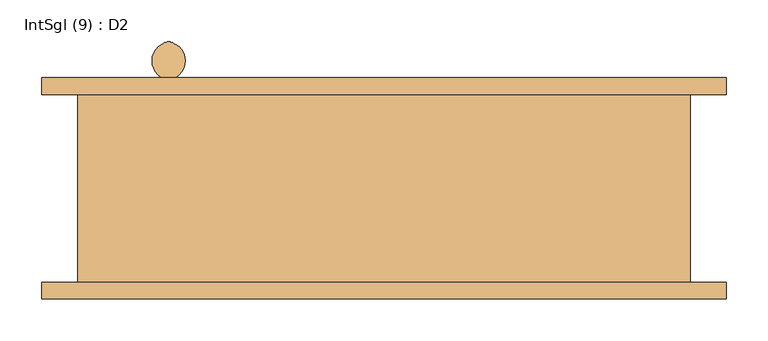
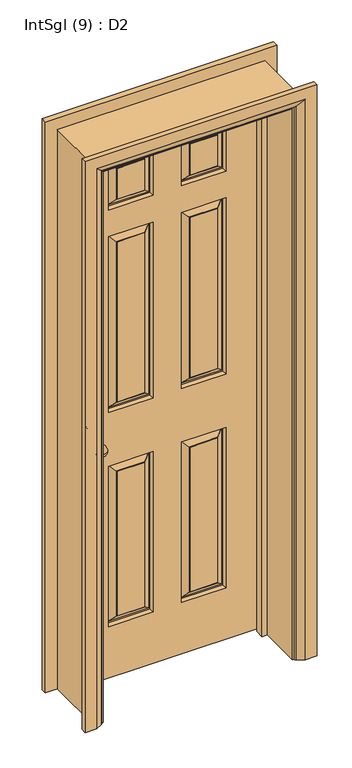
"""IFC4 building model written with IfcOpenShell, lengths in millimetres: door geometry, IntSgl (9) : D2."""

from ifc_helpers import new_model, si_unit, point, frame, origin, place, context, project, spatial, polyline, circle_curve, ellipse_curve, trimmed, outline, extrude, faceted_brep, source, transform, mapped, element, save
from ifc_brep_helpers import plane_surface, cylinder_surface, revolved_surface, advanced_brep


def intsgl_9_d2_5357b631(model_context):
    return source(origin(), model_context, "Body", "SolidModel", [
        advanced_brep(
        [(-253.0, 55.5, 900.0), (-258.0, 11.062589, 900.0), (-263.0, 55.5, 900.0), (-263.0, 70.5, 900.0), (-253.0, 70.5, 900.0), (-278.0, 74.5, 900.0), (-238.0, 74.5, 900.0), (-278.0, 70.5, 900.0), (-238.0, 70.5, 900.0)],
        [
            (0, 1, circle_curve(frame((-261.1884862, 33.9213505, 900.0), z_axis=(0.0, 0.0, -1.0), x_axis=(0.0, 1.0, 0.0)), 23.0800654)),
            (1, 2, circle_curve(frame((-254.8115138, 33.9213505, 900.0), z_axis=(0.0, 0.0, -1.0), x_axis=(0.0, 1.0, 0.0)), 23.0800654)),
            (2, 0, circle_curve(frame((-258.0, 55.5, 900.0), z_axis=(0.0, -1.0, 0.0), x_axis=(-1.0, 0.0, 0.0)), 5.0)),
            (0, 2, circle_curve(frame((-258.0, 55.5, 900.0), z_axis=(0.0, -1.0, 0.0), x_axis=(-1.0, 0.0, 0.0)), 5.0)),
            (2, 3),
            (3, 4, circle_curve(frame((-258.0, 70.5, 900.0), z_axis=(0.0, -1.0, 0.0), x_axis=(-1.0, 0.0, 0.0)), 5.0)),
            (4, 0),
            (4, 3, circle_curve(frame((-258.0, 70.5, 900.0), z_axis=(0.0, -1.0, 0.0), x_axis=(-1.0, 0.0, 0.0)), 5.0)),
            (5, 6, circle_curve(frame((-258.0, 74.5, 900.0), z_axis=(0.0, 1.0, 0.0), x_axis=(1.0, 0.0, 0.0)), 20.0)),
            (6, 5, circle_curve(frame((-258.0, 74.5, 900.0), z_axis=(0.0, 1.0, 0.0), x_axis=(1.0, 0.0, 0.0)), 20.0)),
            (7, 8, circle_curve(frame((-258.0, 70.5, 900.0), z_axis=(0.0, -1.0, 0.0), x_axis=(1.0, 0.0, 0.0)), 20.0)),
            (8, 7, circle_curve(frame((-258.0, 70.5, 900.0), z_axis=(0.0, -1.0, 0.0), x_axis=(1.0, 0.0, 0.0)), 20.0)),
            (6, 8),
            (7, 5),
        ],
        [
            revolved_surface(trimmed(ellipse_curve(frame((-254.8115138, 33.9213505, 900.0), z_axis=(0.0, 0.0, -1.0), x_axis=(0.0, 1.0, 0.0)), 23.0800654, 23.0800654), [point((-258.0, 11.062589, 900.0))], [point((-263.0, 55.5, 900.0))], True, "CARTESIAN"), (-258.0, 70.5, 900.0), (0.0, 1.0, 0.0)),
            cylinder_surface(frame((-258.0, 70.5, 900.0), z_axis=(0.0, 1.0, 0.0), x_axis=(-1.0, 0.0, 0.0)), 5.0),
            plane_surface(frame((-238.0, 74.5, 900.0), z_axis=(0.0, 1.0, 0.0), x_axis=(0.0, 0.0, 1.0))),
            plane_surface(frame((-238.0, 70.5, 900.0), z_axis=(0.0, -1.0, 0.0), x_axis=(0.0, 0.0, -1.0))),
            cylinder_surface(frame((-258.0, 70.5, 900.0), z_axis=(0.0, 1.0, 0.0), x_axis=(1.0, 0.0, 0.0)), 20.0),
        ],
        [
            (0, [[1, 2, 3]]),
            (0, [[-1, 4, -2]]),
            (1, [[5, 6, 7, -3]]),
            (1, [[-7, 8, -5, -4]]),
            (2, [[9, 10]]),
            (3, [[11, 12], [-8, -6]]),
            (4, [[13, -11, 14, -10]]),
            (4, [[-14, -12, -13, -9]]),
        ],
    ),
        advanced_brep(
        [(-253.0, 131.5, 900.0), (-263.0, 131.5, 900.0), (-258.0, 175.937411, 900.0), (-253.0, 116.5, 900.0), (-263.0, 116.5, 900.0), (-278.0, 112.5, 900.0), (-238.0, 112.5, 900.0), (-278.0, 116.5, 900.0), (-238.0, 116.5, 900.0)],
        [
            (0, 1, circle_curve(frame((-258.0, 131.5, 900.0), z_axis=(0.0, 1.0, 0.0), x_axis=(-1.0, 0.0, 0.0)), 5.0)),
            (1, 2, circle_curve(frame((-254.8115138, 153.0786495, 900.0), z_axis=(0.0, 0.0, -1.0), x_axis=(0.0, -1.0, 0.0)), 23.0800654)),
            (2, 0, circle_curve(frame((-261.1884862, 153.0786495, 900.0), z_axis=(0.0, 0.0, -1.0), x_axis=(0.0, -1.0, 0.0)), 23.0800654)),
            (1, 0, circle_curve(frame((-258.0, 131.5, 900.0), z_axis=(0.0, 1.0, 0.0), x_axis=(-1.0, 0.0, 0.0)), 5.0)),
            (0, 3),
            (3, 4, circle_curve(frame((-258.0, 116.5, 900.0), z_axis=(0.0, 1.0, 0.0), x_axis=(-1.0, 0.0, 0.0)), 5.0)),
            (4, 1),
            (4, 3, circle_curve(frame((-258.0, 116.5, 900.0), z_axis=(0.0, 1.0, 0.0), x_axis=(-1.0, 0.0, 0.0)), 5.0)),
            (5, 6, circle_curve(frame((-258.0, 112.5, 900.0), z_axis=(0.0, -1.0, 0.0), x_axis=(1.0, 0.0, 0.0)), 20.0)),
            (6, 5, circle_curve(frame((-258.0, 112.5, 900.0), z_axis=(0.0, -1.0, 0.0), x_axis=(1.0, 0.0, 0.0)), 20.0)),
            (7, 8, circle_curve(frame((-258.0, 116.5, 900.0), z_axis=(0.0, 1.0, 0.0), x_axis=(1.0, 0.0, 0.0)), 20.0)),
            (8, 7, circle_curve(frame((-258.0, 116.5, 900.0), z_axis=(0.0, 1.0, 0.0), x_axis=(1.0, 0.0, 0.0)), 20.0)),
            (5, 7),
            (8, 6),
        ],
        [
            revolved_surface(trimmed(ellipse_curve(frame((-254.8115138, 153.0786495, 900.0), z_axis=(0.0, 0.0, 1.0), x_axis=(0.0, -1.0, 0.0)), 23.0800654, 23.0800654), [point((-258.0, 175.937411, 900.0))], [point((-263.0, 131.5, 900.0))], True, "CARTESIAN"), (-258.0, 116.5, 900.0), (0.0, -1.0, 0.0)),
            cylinder_surface(frame((-258.0, 116.5, 900.0), z_axis=(0.0, -1.0, 0.0), x_axis=(-1.0, 0.0, 0.0)), 5.0),
            plane_surface(frame((-238.0, 112.5, 900.0), z_axis=(0.0, -1.0, 0.0), x_axis=(0.0, 0.0, 1.0))),
            plane_surface(frame((-238.0, 116.5, 900.0), z_axis=(0.0, 1.0, 0.0), x_axis=(0.0, 0.0, -1.0))),
            cylinder_surface(frame((-258.0, 116.5, 900.0), z_axis=(0.0, -1.0, 0.0), x_axis=(1.0, 0.0, 0.0)), 20.0),
        ],
        [
            (0, [[1, 2, 3]]),
            (0, [[-2, 4, -3]]),
            (1, [[-1, 5, 6, 7]]),
            (1, [[-4, -7, 8, -5]]),
            (2, [[9, 10]]),
            (3, [[11, 12], [-6, -8]]),
            (4, [[-9, 13, -12, 14]]),
            (4, [[-10, -14, -11, -13]]),
        ],
    ),
        faceted_brep([(-333.0, 74.5, 2058.0), (-333.0, 74.5, 8.0), (333.0, 74.5, 8.0), (333.0, 74.5, 2058.0), (-50.0, 74.5, 800.0), (-50.0, 74.5, 200.0), (-208.0, 74.5, 200.0), (-208.0, 74.5, 800.0), (208.0, 74.5, 800.0), (208.0, 74.5, 200.0), (50.0, 74.5, 200.0), (50.0, 74.5, 800.0), (-50.0, 74.5, 1658.0), (-50.0, 74.5, 1000.0), (-208.0, 74.5, 1000.0), (-208.0, 74.5, 1658.0), (208.0, 74.5, 1658.0), (208.0, 74.5, 1000.0), (50.0, 74.5, 1000.0), (50.0, 74.5, 1658.0), (-50.0, 74.5, 1933.0), (-50.0, 74.5, 1758.0), (-208.0, 74.5, 1758.0), (-208.0, 74.5, 1933.0), (208.0, 74.5, 1933.0), (208.0, 74.5, 1758.0), (50.0, 74.5, 1758.0), (50.0, 74.5, 1933.0), (-80.0, 74.5, 230.0), (-80.0, 74.5, 770.0), (-178.0, 74.5, 770.0), (-178.0, 74.5, 230.0), (178.0, 74.5, 230.0), (178.0, 74.5, 770.0), (80.0, 74.5, 770.0), (80.0, 74.5, 230.0), (-80.0, 74.5, 1030.0), (-80.0, 74.5, 1628.0), (-178.0, 74.5, 1628.0), (-178.0, 74.5, 1030.0), (178.0, 74.5, 1030.0), (178.0, 74.5, 1628.0), (80.0, 74.5, 1628.0), (80.0, 74.5, 1030.0), (-80.0, 74.5, 1788.0), (-80.0, 74.5, 1903.0), (-178.0, 74.5, 1903.0), (-178.0, 74.5, 1788.0), (178.0, 74.5, 1788.0), (178.0, 74.5, 1903.0), (80.0, 74.5, 1903.0), (80.0, 74.5, 1788.0), (-333.0, 112.5, 2058.0), (333.0, 112.5, 2058.0), (333.0, 112.5, 8.0), (-333.0, 112.5, 8.0), (50.0, 112.5, 800.0), (50.0, 112.5, 200.0), (208.0, 112.5, 200.0), (208.0, 112.5, 800.0), (-208.0, 112.5, 800.0), (-208.0, 112.5, 200.0), (-50.0, 112.5, 200.0), (-50.0, 112.5, 800.0), (50.0, 112.5, 1658.0), (50.0, 112.5, 1000.0), (208.0, 112.5, 1000.0), (208.0, 112.5, 1658.0), (-208.0, 112.5, 1658.0), (-208.0, 112.5, 1000.0), (-50.0, 112.5, 1000.0), (-50.0, 112.5, 1658.0), (50.0, 112.5, 1933.0), (50.0, 112.5, 1758.0), (208.0, 112.5, 1758.0), (208.0, 112.5, 1933.0), (-208.0, 112.5, 1933.0), (-208.0, 112.5, 1758.0), (-50.0, 112.5, 1758.0), (-50.0, 112.5, 1933.0), (80.0, 112.5, 230.0), (80.0, 112.5, 770.0), (178.0, 112.5, 770.0), (178.0, 112.5, 230.0), (-178.0, 112.5, 230.0), (-178.0, 112.5, 770.0), (-80.0, 112.5, 770.0), (-80.0, 112.5, 230.0), (80.0, 112.5, 1030.0), (80.0, 112.5, 1628.0), (178.0, 112.5, 1628.0), (178.0, 112.5, 1030.0), (-178.0, 112.5, 1030.0), (-178.0, 112.5, 1628.0), (-80.0, 112.5, 1628.0), (-80.0, 112.5, 1030.0), (80.0, 112.5, 1788.0), (80.0, 112.5, 1903.0), (178.0, 112.5, 1903.0), (178.0, 112.5, 1788.0), (-178.0, 112.5, 1788.0), (-178.0, 112.5, 1903.0), (-80.0, 112.5, 1903.0), (-80.0, 112.5, 1788.0), (80.0, 111.5, 230.0), (80.0, 111.5, 770.0), (58.0, 97.5, 208.0), (58.0, 97.5, 792.0), (78.0, 111.5, 772.0), (78.0, 111.5, 228.0), (53.0, 97.5, 797.0), (53.0, 97.5, 203.0), (178.0, 111.5, 770.0), (200.0, 97.5, 792.0), (180.0, 111.5, 772.0), (205.0, 97.5, 797.0), (178.0, 111.5, 230.0), (200.0, 97.5, 208.0), (180.0, 111.5, 228.0), (205.0, 97.5, 203.0), (-178.0, 111.5, 230.0), (-178.0, 111.5, 770.0), (-200.0, 97.5, 208.0), (-200.0, 97.5, 792.0), (-180.0, 111.5, 772.0), (-180.0, 111.5, 228.0), (-205.0, 97.5, 797.0), (-205.0, 97.5, 203.0), (-80.0, 111.5, 770.0), (-58.0, 97.5, 792.0), (-78.0, 111.5, 772.0), (-53.0, 97.5, 797.0), (-80.0, 111.5, 230.0), (-58.0, 97.5, 208.0), (-78.0, 111.5, 228.0), (-53.0, 97.5, 203.0), (80.0, 111.5, 1030.0), (80.0, 111.5, 1628.0), (58.0, 97.5, 1008.0), (58.0, 97.5, 1650.0), (78.0, 111.5, 1630.0), (78.0, 111.5, 1028.0), (53.0, 97.5, 1655.0), (53.0, 97.5, 1003.0), (178.0, 111.5, 1628.0), (200.0, 97.5, 1650.0), (180.0, 111.5, 1630.0), (205.0, 97.5, 1655.0), (178.0, 111.5, 1030.0), (200.0, 97.5, 1008.0), (180.0, 111.5, 1028.0), (205.0, 97.5, 1003.0), (-178.0, 111.5, 1030.0), (-178.0, 111.5, 1628.0), (-200.0, 97.5, 1008.0), (-200.0, 97.5, 1650.0), (-180.0, 111.5, 1630.0), (-180.0, 111.5, 1028.0), (-205.0, 97.5, 1655.0), (-205.0, 97.5, 1003.0), (-80.0, 111.5, 1628.0), (-58.0, 97.5, 1650.0), (-78.0, 111.5, 1630.0), (-53.0, 97.5, 1655.0), (-80.0, 111.5, 1030.0), (-58.0, 97.5, 1008.0), (-78.0, 111.5, 1028.0), (-53.0, 97.5, 1003.0), (80.0, 111.5, 1788.0), (80.0, 111.5, 1903.0), (58.0, 97.5, 1766.0), (58.0, 97.5, 1925.0), (78.0, 111.5, 1905.0), (78.0, 111.5, 1786.0), (53.0, 97.5, 1930.0), (53.0, 97.5, 1761.0), (178.0, 111.5, 1903.0), (200.0, 97.5, 1925.0), (180.0, 111.5, 1905.0), (205.0, 97.5, 1930.0), (178.0, 111.5, 1788.0), (200.0, 97.5, 1766.0), (180.0, 111.5, 1786.0), (205.0, 97.5, 1761.0), (-178.0, 111.5, 1788.0), (-178.0, 111.5, 1903.0), (-200.0, 97.5, 1766.0), (-200.0, 97.5, 1925.0), (-180.0, 111.5, 1905.0), (-180.0, 111.5, 1786.0), (-205.0, 97.5, 1930.0), (-205.0, 97.5, 1761.0), (-80.0, 111.5, 1903.0), (-58.0, 97.5, 1925.0), (-78.0, 111.5, 1905.0), (-53.0, 97.5, 1930.0), (-80.0, 111.5, 1788.0), (-58.0, 97.5, 1766.0), (-78.0, 111.5, 1786.0), (-53.0, 97.5, 1761.0), (-80.0, 75.5, 230.0), (-80.0, 75.5, 770.0), (-58.0, 89.5, 208.0), (-58.0, 89.5, 792.0), (-78.0, 75.5, 772.0), (-78.0, 75.5, 228.0), (-53.0, 89.5, 797.0), (-53.0, 89.5, 203.0), (-178.0, 75.5, 770.0), (-200.0, 89.5, 792.0), (-180.0, 75.5, 772.0), (-205.0, 89.5, 797.0), (-178.0, 75.5, 230.0), (-200.0, 89.5, 208.0), (-180.0, 75.5, 228.0), (-205.0, 89.5, 203.0), (178.0, 75.5, 230.0), (178.0, 75.5, 770.0), (200.0, 89.5, 208.0), (200.0, 89.5, 792.0), (180.0, 75.5, 772.0), (180.0, 75.5, 228.0), (205.0, 89.5, 797.0), (205.0, 89.5, 203.0), (80.0, 75.5, 770.0), (58.0, 89.5, 792.0), (78.0, 75.5, 772.0), (53.0, 89.5, 797.0), (80.0, 75.5, 230.0), (58.0, 89.5, 208.0), (78.0, 75.5, 228.0), (53.0, 89.5, 203.0), (-80.0, 75.5, 1030.0), (-80.0, 75.5, 1628.0), (-58.0, 89.5, 1008.0), (-58.0, 89.5, 1650.0), (-78.0, 75.5, 1630.0), (-78.0, 75.5, 1028.0), (-53.0, 89.5, 1655.0), (-53.0, 89.5, 1003.0), (-178.0, 75.5, 1628.0), (-200.0, 89.5, 1650.0), (-180.0, 75.5, 1630.0), (-205.0, 89.5, 1655.0), (-178.0, 75.5, 1030.0), (-200.0, 89.5, 1008.0), (-180.0, 75.5, 1028.0), (-205.0, 89.5, 1003.0), (178.0, 75.5, 1030.0), (178.0, 75.5, 1628.0), (200.0, 89.5, 1008.0), (200.0, 89.5, 1650.0), (180.0, 75.5, 1630.0), (180.0, 75.5, 1028.0), (205.0, 89.5, 1655.0), (205.0, 89.5, 1003.0), (80.0, 75.5, 1628.0), (58.0, 89.5, 1650.0), (78.0, 75.5, 1630.0), (53.0, 89.5, 1655.0), (80.0, 75.5, 1030.0), (58.0, 89.5, 1008.0), (78.0, 75.5, 1028.0), (53.0, 89.5, 1003.0), (-80.0, 75.5, 1788.0), (-80.0, 75.5, 1903.0), (-58.0, 89.5, 1766.0), (-58.0, 89.5, 1925.0), (-78.0, 75.5, 1905.0), (-78.0, 75.5, 1786.0), (-53.0, 89.5, 1930.0), (-53.0, 89.5, 1761.0), (-178.0, 75.5, 1903.0), (-200.0, 89.5, 1925.0), (-180.0, 75.5, 1905.0), (-205.0, 89.5, 1930.0), (-178.0, 75.5, 1788.0), (-200.0, 89.5, 1766.0), (-180.0, 75.5, 1786.0), (-205.0, 89.5, 1761.0), (178.0, 75.5, 1788.0), (178.0, 75.5, 1903.0), (200.0, 89.5, 1766.0), (200.0, 89.5, 1925.0), (180.0, 75.5, 1905.0), (180.0, 75.5, 1786.0), (205.0, 89.5, 1930.0), (205.0, 89.5, 1761.0), (80.0, 75.5, 1903.0), (58.0, 89.5, 1925.0), (78.0, 75.5, 1905.0), (53.0, 89.5, 1930.0), (80.0, 75.5, 1788.0), (58.0, 89.5, 1766.0), (78.0, 75.5, 1786.0), (53.0, 89.5, 1761.0)], [[[0, 1, 2, 3], [4, 5, 6, 7], [8, 9, 10, 11], [12, 13, 14, 15], [16, 17, 18, 19], [20, 21, 22, 23], [24, 25, 26, 27]], [[28, 29, 30, 31]], [[32, 33, 34, 35]], [[36, 37, 38, 39]], [[40, 41, 42, 43]], [[44, 45, 46, 47]], [[48, 49, 50, 51]], [[52, 53, 54, 55], [56, 57, 58, 59], [60, 61, 62, 63], [64, 65, 66, 67], [68, 69, 70, 71], [72, 73, 74, 75], [76, 77, 78, 79]], [[80, 81, 82, 83]], [[84, 85, 86, 87]], [[88, 89, 90, 91]], [[92, 93, 94, 95]], [[96, 97, 98, 99]], [[100, 101, 102, 103]], [[1, 0, 52, 55]], [[2, 1, 55, 54]], [[3, 2, 54, 53]], [[0, 3, 53, 52]], [[104, 105, 81, 80]], [[106, 107, 108, 109]], [[56, 110, 111, 57]], [[81, 105, 112, 82]], [[108, 107, 113, 114]], [[110, 56, 59, 115]], [[82, 112, 116, 83]], [[114, 113, 117, 118]], [[115, 59, 58, 119]], [[104, 80, 83, 116]], [[109, 108, 114, 118], [105, 104, 116, 112]], [[106, 109, 118, 117]], [[111, 110, 115, 119], [107, 106, 117, 113]], [[57, 111, 119, 58]], [[120, 121, 85, 84]], [[122, 123, 124, 125]], [[60, 126, 127, 61]], [[85, 121, 128, 86]], [[124, 123, 129, 130]], [[126, 60, 63, 131]], [[86, 128, 132, 87]], [[130, 129, 133, 134]], [[131, 63, 62, 135]], [[120, 84, 87, 132]], [[125, 124, 130, 134], [121, 120, 132, 128]], [[122, 125, 134, 133]], [[127, 126, 131, 135], [123, 122, 133, 129]], [[61, 127, 135, 62]], [[136, 137, 89, 88]], [[138, 139, 140, 141]], [[64, 142, 143, 65]], [[89, 137, 144, 90]], [[140, 139, 145, 146]], [[142, 64, 67, 147]], [[90, 144, 148, 91]], [[146, 145, 149, 150]], [[147, 67, 66, 151]], [[136, 88, 91, 148]], [[141, 140, 146, 150], [137, 136, 148, 144]], [[138, 141, 150, 149]], [[143, 142, 147, 151], [139, 138, 149, 145]], [[65, 143, 151, 66]], [[152, 153, 93, 92]], [[154, 155, 156, 157]], [[68, 158, 159, 69]], [[93, 153, 160, 94]], [[156, 155, 161, 162]], [[158, 68, 71, 163]], [[94, 160, 164, 95]], [[162, 161, 165, 166]], [[163, 71, 70, 167]], [[152, 92, 95, 164]], [[157, 156, 162, 166], [153, 152, 164, 160]], [[154, 157, 166, 165]], [[159, 158, 163, 167], [155, 154, 165, 161]], [[69, 159, 167, 70]], [[168, 169, 97, 96]], [[170, 171, 172, 173]], [[72, 174, 175, 73]], [[97, 169, 176, 98]], [[172, 171, 177, 178]], [[174, 72, 75, 179]], [[98, 176, 180, 99]], [[178, 177, 181, 182]], [[179, 75, 74, 183]], [[168, 96, 99, 180]], [[173, 172, 178, 182], [169, 168, 180, 176]], [[170, 173, 182, 181]], [[175, 174, 179, 183], [171, 170, 181, 177]], [[73, 175, 183, 74]], [[184, 185, 101, 100]], [[186, 187, 188, 189]], [[76, 190, 191, 77]], [[101, 185, 192, 102]], [[188, 187, 193, 194]], [[190, 76, 79, 195]], [[102, 192, 196, 103]], [[194, 193, 197, 198]], [[195, 79, 78, 199]], [[184, 100, 103, 196]], [[189, 188, 194, 198], [185, 184, 196, 192]], [[186, 189, 198, 197]], [[191, 190, 195, 199], [187, 186, 197, 193]], [[77, 191, 199, 78]], [[200, 201, 29, 28]], [[202, 203, 204, 205]], [[4, 206, 207, 5]], [[29, 201, 208, 30]], [[204, 203, 209, 210]], [[206, 4, 7, 211]], [[30, 208, 212, 31]], [[210, 209, 213, 214]], [[211, 7, 6, 215]], [[200, 28, 31, 212]], [[205, 204, 210, 214], [201, 200, 212, 208]], [[202, 205, 214, 213]], [[207, 206, 211, 215], [203, 202, 213, 209]], [[5, 207, 215, 6]], [[216, 217, 33, 32]], [[218, 219, 220, 221]], [[8, 222, 223, 9]], [[33, 217, 224, 34]], [[220, 219, 225, 226]], [[222, 8, 11, 227]], [[34, 224, 228, 35]], [[226, 225, 229, 230]], [[227, 11, 10, 231]], [[216, 32, 35, 228]], [[221, 220, 226, 230], [217, 216, 228, 224]], [[218, 221, 230, 229]], [[223, 222, 227, 231], [219, 218, 229, 225]], [[9, 223, 231, 10]], [[232, 233, 37, 36]], [[234, 235, 236, 237]], [[12, 238, 239, 13]], [[37, 233, 240, 38]], [[236, 235, 241, 242]], [[238, 12, 15, 243]], [[38, 240, 244, 39]], [[242, 241, 245, 246]], [[243, 15, 14, 247]], [[232, 36, 39, 244]], [[237, 236, 242, 246], [233, 232, 244, 240]], [[234, 237, 246, 245]], [[239, 238, 243, 247], [235, 234, 245, 241]], [[13, 239, 247, 14]], [[248, 249, 41, 40]], [[250, 251, 252, 253]], [[16, 254, 255, 17]], [[41, 249, 256, 42]], [[252, 251, 257, 258]], [[254, 16, 19, 259]], [[42, 256, 260, 43]], [[258, 257, 261, 262]], [[259, 19, 18, 263]], [[248, 40, 43, 260]], [[253, 252, 258, 262], [249, 248, 260, 256]], [[250, 253, 262, 261]], [[255, 254, 259, 263], [251, 250, 261, 257]], [[17, 255, 263, 18]], [[264, 265, 45, 44]], [[266, 267, 268, 269]], [[20, 270, 271, 21]], [[45, 265, 272, 46]], [[268, 267, 273, 274]], [[270, 20, 23, 275]], [[46, 272, 276, 47]], [[274, 273, 277, 278]], [[275, 23, 22, 279]], [[264, 44, 47, 276]], [[269, 268, 274, 278], [265, 264, 276, 272]], [[266, 269, 278, 277]], [[271, 270, 275, 279], [267, 266, 277, 273]], [[21, 271, 279, 22]], [[280, 281, 49, 48]], [[282, 283, 284, 285]], [[24, 286, 287, 25]], [[49, 281, 288, 50]], [[284, 283, 289, 290]], [[286, 24, 27, 291]], [[50, 288, 292, 51]], [[290, 289, 293, 294]], [[291, 27, 26, 295]], [[280, 48, 51, 292]], [[285, 284, 290, 294], [281, 280, 292, 288]], [[282, 285, 294, 293]], [[287, 286, 291, 295], [283, 282, 293, 289]], [[25, 287, 295, 26]]]),
        faceted_brep([(-335.0, 112.5, 0.0), (-335.0, -112.5, 0.0), (-367.0, -112.5, 0.0), (-367.0, 112.5, 0.0), (-335.0, 112.5, 2060.0), (-335.0, -112.5, 2060.0), (-367.0, -112.5, 2092.0), (-367.0, 112.5, 2092.0), (335.0, 112.5, 0.0), (367.0, 112.5, 0.0), (367.0, -112.5, 0.0), (335.0, -112.5, 0.0), (335.0, 112.5, 2060.0), (367.0, 112.5, 2092.0), (367.0, -112.5, 2092.0), (335.0, -112.5, 2060.0)], [[[0, 1, 2, 3]], [[1, 0, 4, 5]], [[2, 1, 5, 6]], [[3, 2, 6, 7]], [[0, 3, 7, 4]], [[8, 9, 10, 11]], [[12, 13, 9, 8]], [[13, 14, 10, 9]], [[14, 15, 11, 10]], [[15, 12, 8, 11]], [[5, 4, 12, 15]], [[6, 5, 15, 14]], [[7, 6, 14, 13]], [[4, 7, 13, 12]]]),
        extrude(outline(polyline([(0.0, -335.0), (0.0, -316.0), (2041.0, -316.0), (2041.0, 316.0), (0.0, 316.0), (0.0, 335.0), (2060.0, 335.0), (2060.0, -335.0), (0.0, -335.0)])), frame((0.0, 40.5, 0.0), z_axis=(0.0, 1.0, 0.0), x_axis=(0.0, 0.0, 1.0)), (0.0, 0.0, 1.0), 32.0),
        advanced_brep(
        [(-410.0, -132.5, 0.0), (-410.0, -112.5, 0.0), (-340.0, -112.5, 0.0), (-344.0, -118.5, 0.0), (-370.0, -132.5, 0.0), (-410.0, -132.5, 2135.0), (-410.0, -112.5, 2135.0), (410.0, -112.5, 2135.0), (410.0, -112.5, 0.0), (340.0, -112.5, 0.0), (340.0, -112.5, 2065.0), (-340.0, -112.5, 2065.0), (-344.0, -118.5, 2069.0), (-370.0, -132.5, 2095.0), (370.0, -132.5, 2095.0), (370.0, -132.5, 0.0), (410.0, -132.5, 0.0), (410.0, -132.5, 2135.0), (344.0, -118.5, 0.0), (344.0, -118.5, 2069.0)],
        [
            (0, 1),
            (1, 2),
            (2, 3, circle_curve(frame((-348.0, -111.5, 0.0), z_axis=(0.0, 0.0, -1.0), x_axis=(-1.0, 0.0, 0.0)), 8.0622577)),
            (3, 4),
            (4, 0),
            (0, 5),
            (5, 6),
            (6, 1),
            (6, 7),
            (7, 8),
            (8, 9),
            (9, 10),
            (10, 11),
            (11, 2),
            (11, 12, ellipse_curve(frame((-348.0, -111.5, 2073.0), z_axis=(-0.7071067811865475, 0.0, -0.7071067811865475), x_axis=(0.7071067811865474, 0.0, -0.7071067811865476)), 11.4017543, 8.0622577)),
            (12, 3),
            (12, 13),
            (13, 4),
            (13, 14),
            (14, 15),
            (15, 16),
            (16, 17),
            (17, 5),
            (7, 17),
            (16, 8),
            (15, 18),
            (18, 9, circle_curve(frame((348.0, -111.5, 0.0), z_axis=(0.0, 0.0, -1.0), x_axis=(1.0, 0.0, 0.0)), 8.0622577)),
            (19, 10, ellipse_curve(frame((348.0, -111.5, 2073.0), z_axis=(0.7071067811865475, 0.0, -0.7071067811865475), x_axis=(0.7071067811865474, 0.0, 0.7071067811865476)), 11.4017543, 8.0622577)),
            (18, 19),
            (14, 19),
            (19, 12),
        ],
        [
            plane_surface(frame((-340.0, -112.5, 0.0), z_axis=(0.0, 0.0, -1.0), x_axis=(0.0, -1.0, 0.0))),
            plane_surface(frame((-410.0, -132.5, 0.0), z_axis=(-1.0, 0.0, 0.0), x_axis=(0.0, 0.0, 1.0))),
            plane_surface(frame((-410.0, -112.5, 0.0), z_axis=(0.0, 1.0, 0.0), x_axis=(0.0, 0.0, 1.0))),
            cylinder_surface(frame((-348.0, -111.5, 0.0), z_axis=(0.0, 0.0, -1.0), x_axis=(-1.0, 0.0, 0.0)), 8.0622577),
            plane_surface(frame((-344.0, -118.5, 0.0), z_axis=(0.4740998230350183, -0.8804710999221749, 0.0), x_axis=(0.0, 0.0, 1.0))),
            plane_surface(frame((-370.0, -132.5, 0.0), z_axis=(0.0, -1.0, 0.0), x_axis=(0.0, 0.0, 1.0))),
            plane_surface(frame((410.0, -132.5, 2135.0), z_axis=(1.0, 0.0, 0.0), x_axis=(0.0, 0.0, -1.0))),
            plane_surface(frame((340.0, -112.5, 0.0), z_axis=(0.0, 0.0, -1.0), x_axis=(0.0, -1.0, 0.0))),
            cylinder_surface(frame((348.0, -111.5, 2065.0), z_axis=(0.0, 0.0, 1.0), x_axis=(1.0, 0.0, 0.0)), 8.0622577),
            plane_surface(frame((344.0, -118.5, 2069.0), z_axis=(-0.4740998230350183, -0.8804710999221749, 0.0), x_axis=(0.0, 0.0, -1.0))),
            plane_surface(frame((-410.0, -132.5, 2135.0), z_axis=(0.0, 0.0, 1.0), x_axis=(1.0, 0.0, 0.0))),
            cylinder_surface(frame((-340.0, -111.5, 2073.0), z_axis=(-1.0, 0.0, 0.0), x_axis=(0.0, 0.0, 1.0)), 8.0622577),
            plane_surface(frame((-344.0, -118.5, 2069.0), z_axis=(0.0, -0.8804710999221749, -0.4740998230350183), x_axis=(1.0, 0.0, 0.0))),
        ],
        [
            (0, [[1, 2, 3, 4, 5]]),
            (1, [[-1, 6, 7, 8]]),
            (2, [[-2, -8, 9, 10, 11, 12, 13, 14]]),
            (3, [[-3, -14, 15, 16]]),
            (4, [[-4, -16, 17, 18]]),
            (5, [[-5, -18, 19, 20, 21, 22, 23, -6]]),
            (6, [[24, -22, 25, -10]]),
            (7, [[-21, 26, 27, -11, -25]]),
            (8, [[28, -12, -27, 29]]),
            (9, [[30, -29, -26, -20]]),
            (10, [[-7, -23, -24, -9]]),
            (11, [[-15, -13, -28, 31]]),
            (12, [[-17, -31, -30, -19]]),
        ],
    ),
        advanced_brep(
        [(410.0, 132.5, 0.0), (410.0, 112.5, 0.0), (340.0, 112.5, 0.0), (344.0, 118.5, 0.0), (370.0, 132.5, 0.0), (410.0, 132.5, 2135.0), (410.0, 112.5, 2135.0), (-410.0, 112.5, 2135.0), (-410.0, 112.5, 0.0), (-340.0, 112.5, 0.0), (-340.0, 112.5, 2065.0), (340.0, 112.5, 2065.0), (344.0, 118.5, 2069.0), (370.0, 132.5, 2095.0), (-370.0, 132.5, 2095.0), (-370.0, 132.5, 0.0), (-410.0, 132.5, 0.0), (-410.0, 132.5, 2135.0), (-344.0, 118.5, 0.0), (-344.0, 118.5, 2069.0)],
        [
            (0, 1),
            (1, 2),
            (2, 3, circle_curve(frame((348.0, 111.5, 0.0), z_axis=(0.0, 0.0, -1.0), x_axis=(1.0, 0.0, 0.0)), 8.0622577)),
            (3, 4),
            (4, 0),
            (0, 5),
            (5, 6),
            (6, 1),
            (6, 7),
            (7, 8),
            (8, 9),
            (9, 10),
            (10, 11),
            (11, 2),
            (11, 12, ellipse_curve(frame((348.0, 111.5, 2073.0), z_axis=(0.7071067811865475, 0.0, -0.7071067811865475), x_axis=(-0.7071067811865474, 0.0, -0.7071067811865476)), 11.4017543, 8.0622577)),
            (12, 3),
            (12, 13),
            (13, 4),
            (13, 14),
            (14, 15),
            (15, 16),
            (16, 17),
            (17, 5),
            (7, 17),
            (16, 8),
            (15, 18),
            (18, 9, circle_curve(frame((-348.0, 111.5, 0.0), z_axis=(0.0, 0.0, -1.0), x_axis=(-1.0, 0.0, 0.0)), 8.0622577)),
            (19, 10, ellipse_curve(frame((-348.0, 111.5, 2073.0), z_axis=(-0.7071067811865475, 0.0, -0.7071067811865475), x_axis=(-0.7071067811865474, 0.0, 0.7071067811865476)), 11.4017543, 8.0622577)),
            (18, 19),
            (14, 19),
            (19, 12),
        ],
        [
            plane_surface(frame((340.0, 112.5, 0.0), z_axis=(0.0, 0.0, -1.0), x_axis=(0.0, 1.0, 0.0))),
            plane_surface(frame((410.0, 132.5, 0.0), z_axis=(1.0, 0.0, 0.0), x_axis=(0.0, 0.0, 1.0))),
            plane_surface(frame((410.0, 112.5, 0.0), z_axis=(0.0, -1.0, 0.0), x_axis=(0.0, 0.0, 1.0))),
            cylinder_surface(frame((348.0, 111.5, 0.0), z_axis=(0.0, 0.0, -1.0), x_axis=(1.0, 0.0, 0.0)), 8.0622577),
            plane_surface(frame((344.0, 118.5, 0.0), z_axis=(-0.4740998230350183, 0.8804710999221749, 0.0), x_axis=(0.0, 0.0, 1.0))),
            plane_surface(frame((370.0, 132.5, 0.0), z_axis=(0.0, 1.0, 0.0), x_axis=(0.0, 0.0, 1.0))),
            plane_surface(frame((-410.0, 132.5, 2135.0), z_axis=(-1.0, 0.0, 0.0), x_axis=(0.0, 0.0, -1.0))),
            plane_surface(frame((-340.0, 112.5, 0.0), z_axis=(0.0, 0.0, -1.0), x_axis=(0.0, 1.0, 0.0))),
            cylinder_surface(frame((-348.0, 111.5, 2065.0), z_axis=(0.0, 0.0, 1.0), x_axis=(-1.0, 0.0, 0.0)), 8.0622577),
            plane_surface(frame((-344.0, 118.5, 2069.0), z_axis=(0.4740998230350183, 0.8804710999221749, 0.0), x_axis=(0.0, 0.0, -1.0))),
            plane_surface(frame((410.0, 132.5, 2135.0), z_axis=(0.0, 0.0, 1.0), x_axis=(-1.0, 0.0, 0.0))),
            cylinder_surface(frame((340.0, 111.5, 2073.0), z_axis=(1.0, 0.0, 0.0), x_axis=(0.0, 0.0, 1.0)), 8.0622577),
            plane_surface(frame((344.0, 118.5, 2069.0), z_axis=(0.0, 0.8804710999221749, -0.4740998230350183), x_axis=(-1.0, 0.0, 0.0))),
        ],
        [
            (0, [[1, 2, 3, 4, 5]]),
            (1, [[-1, 6, 7, 8]]),
            (2, [[-2, -8, 9, 10, 11, 12, 13, 14]]),
            (3, [[-3, -14, 15, 16]]),
            (4, [[-4, -16, 17, 18]]),
            (5, [[-5, -18, 19, 20, 21, 22, 23, -6]]),
            (6, [[24, -22, 25, -10]]),
            (7, [[-21, 26, 27, -11, -25]]),
            (8, [[28, -12, -27, 29]]),
            (9, [[30, -29, -26, -20]]),
            (10, [[-7, -23, -24, -9]]),
            (11, [[-15, -13, -28, 31]]),
            (12, [[-17, -31, -30, -19]]),
        ],
    ),
    ])


if __name__ == "__main__":
    model = new_model("IFC4")
    model_context = context("Model", 3, world=origin())
    ifc_project = project(units=[si_unit("LENGTHUNIT", "METRE", prefix="MILLI")], contexts=[model_context])
    site = spatial("IfcSite", under=ifc_project)
    building = spatial("IfcBuilding", under=site)
    placement = place(None, origin())
    intsgl_9_d2_shape = intsgl_9_d2_5357b631(model_context)
    element("IfcDoor", 1, ObjectType="IntSgl (9) : D2", at=placement, inside=building, context=model_context, shape_type="MappedRepresentation", body=[
        mapped(intsgl_9_d2_shape, transform((0.0, 0.0, 0.0), x_axis=(1.0, 0.0, 0.0), y_axis=(0.0, 1.0, 0.0), z_axis=(0.0, 0.0, 1.0))),
    ])
    save(model, "model.ifc")

# Revit data of these elements
# Type "IntSgl (9) : D2"
#   Type Mark = "50"
#   Operation = "SingleSwingRight"
#   Manufacturer = "Revit"
#   Keynote = "L20"
#   UnderCut = 8 mm
#   Tolerance = 2 mm
#   Thickness = 38 mm
#   Structural Tolerance = 8 mm
#   StopDepth = 32 mm
#   Stop Thickness = 19 mm
#   Stile Top Rail = 125 mm
#   Stile Shutting = 125 mm
#   Stile Muntin Rail = 100 mm
#   Stile Lock Rail = 200 mm
#   Stile Intermediate/Frieze = 100 mm
#   Stile Hanging = 125 mm
#   Stile Bottom Rail = 200 mm
#   Rough Width = 750 mm
#   Rough Height = 2100 mm
#   Height to Top Lock Rail = 1000 mm
#   Handle Z Distance = 900 mm
#   Handle X Distance = 75 mm
#   Frame Thickness = 32 mm
#   Door Panel Width = 666 mm
#   Height = 2100 mm
#   Width = 750 mm
#   Door Panel Thickness = 38 mm
#   Door Panel Offset = 0 mm
#   Door Panel Height = 2050 mm
#   Architrave Setback = 5 mm
#   Vis - Ironmongery = yes
#   Material Ironmongery = Door - Handle
#   Material Frame = Door - Frame/Mullion
#   Material Door = Door - Panel
#   Material Architrave = Door - Architrave
#   Function = (empty or 0)
#   Wall Closure = (empty or 0)
# Element 1 (IfcDoor, "IntSgl (9) : D2")
#   Materials on its faces: "Door - Panel", "Door - Architrave", "Door - Frame/Mullion", "Door - Handle"
# Materials
#   "Door - Handle": colour RGB 247 247 247, transparency 0
#   "Door - Frame/Mullion": colour RGB 212 179 113, transparency 0
#   "Door - Panel": colour RGB 154 90 5, transparency 0
#   "Door - Architrave": colour RGB 154 90 5, transparency 0
